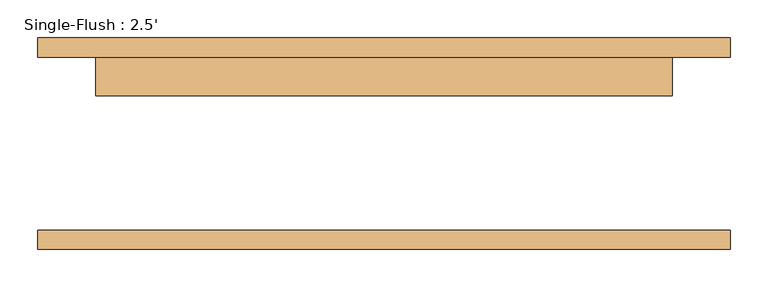
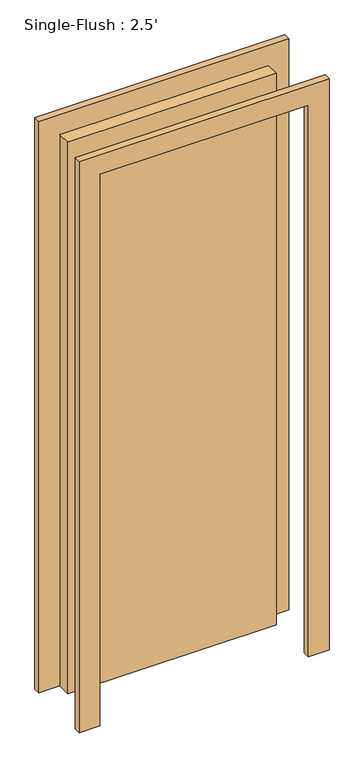
"""IFC4 building model written with IfcOpenShell, lengths in millimetres: door geometry, Single-Flush : 2.5'."""

from ifc_helpers import new_model, si_unit, frame, origin, origin_with_axes, place, context, project, spatial, polyline, outline, extrude, source, transform, mapped, element, save


def single_flush_2_5_bb98abfd(model_context):
    return source(origin(), model_context, "Body", "SweptSolid", [
        extrude(outline(polyline([(2209.8, -457.2), (0.0, -457.2), (0.0, -381.0), (2133.6, -381.0), (2133.6, 381.0), (0.0, 381.0), (0.0, 457.2), (2209.8, 457.2), (2209.8, -457.2)])), frame((0.0, 114.3, 0.0), z_axis=(0.0, 1.0, 0.0), x_axis=(0.0, 0.0, 1.0)), (0.0, 0.0, 1.0), 25.4),
        extrude(outline(polyline([(2209.8, 457.2), (2209.8, -457.2), (0.0, -457.2), (0.0, -381.0), (2133.6, -381.0), (2133.6, 381.0), (0.0, 381.0), (0.0, 457.2), (2209.8, 457.2)])), frame((0.0, -139.7, 0.0), z_axis=(0.0, 1.0, 0.0), x_axis=(0.0, 0.0, 1.0)), (0.0, 0.0, 1.0), 25.4),
        extrude(outline(polyline([(381.0, 63.5), (-381.0, 63.5), (-381.0, 114.3), (381.0, 114.3), (381.0, 63.5)])), origin_with_axes(), (0.0, 0.0, 1.0), 2133.6),
    ])


if __name__ == "__main__":
    model = new_model("IFC4")
    model_context = context("Model", 3, world=origin())
    ifc_project = project(units=[si_unit("LENGTHUNIT", "METRE", prefix="MILLI")], contexts=[model_context])
    site = spatial("IfcSite", under=ifc_project)
    building = spatial("IfcBuilding", under=site)
    placement = place(None, origin())
    single_flush_2_5_shape = single_flush_2_5_bb98abfd(model_context)
    element("IfcDoor", 1, ObjectType="Single-Flush : 2.5'", at=placement, inside=building, context=model_context, shape_type="MappedRepresentation", body=[
        mapped(single_flush_2_5_shape, transform((0.0, 0.0, 0.0), x_axis=(1.0, 0.0, 0.0), y_axis=(0.0, 1.0, 0.0), z_axis=(0.0, 0.0, 1.0))),
    ])
    save(model, "model.ifc")

# Revit data of these elements
# Type "Single-Flush : 2.5'"
#   Type Mark = "8"
#   Construction Type Id = "MDOOR"
#   Assembly Code = "C1020"
#   Analytic Construction = "Metal"
#   Thickness = 0' - 2"
#   Heat Transfer Coefficient (U) = 0.651978 BTU/(h·ft²·°F)
#   Height = 7' - 0"
#   Trim Projection Ext = 0' - 1"
#   Trim Projection Int = 0' - 1"
#   Trim Width = 0' - 3"
#   Width = 2' - 6"
#   Define Thermal Properties by = 1
#   Door Material = Door - Panel
#   Frame Material = Door - Frame
#   Visual Light Transmittance = 0
#   Solar Heat Gain Coefficient = 0
#   Function = (empty or 0)
#   Wall Closure = (empty or 0)
# Element 1 (IfcDoor, "Single-Flush : 2.5'")
#   Materials on its faces: "Door - Frame", "Door - Panel"
# Materials
#   "Door - Panel": class "Wood", colour RGB 210 159 95, transparency 0
#   "Door - Frame": colour RGB 118 70 51, transparency 0
